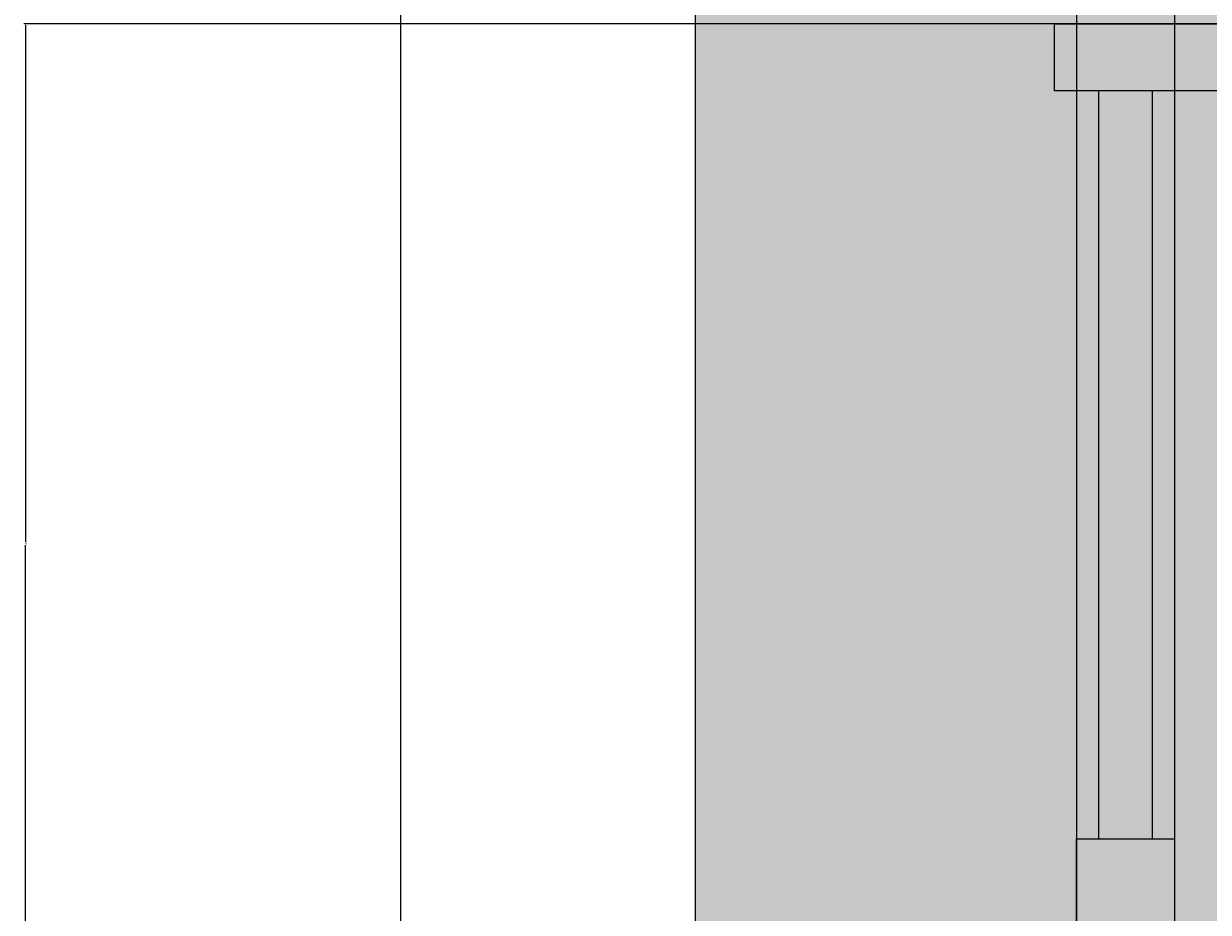
# Model space of a CAD drawing. Units: inches. Extents: x 3024 to 4744, y 1110 to 2100.
# Tile 3 of 29: x 3024 to 3168, y 1294 to 1402. Entities that reach past the tile are written whole.
import ezdxf

# ---------------------------------------------------------------- set-up
doc = ezdxf.new("R2010")
doc.units = ezdxf.units.IN
for name, color, linetype, lineweight in [('A-ANNO-DIMS', 2, 'Continuous', 18), ('A-ELEV', 7, 'Continuous', 25), ('A-ELEV-PATT', 252, 'Continuous', 13), ('A-GLAZ', 4, 'Continuous', 18)]:
    doc.layers.add(name, color=color, linetype=linetype, lineweight=lineweight)
doc.styles.get("Standard").update_dxf_attribs({"font": 'arial.ttf'})
doc.dimstyles.get("Standard").update_dxf_attribs({"dimtxt": 0.18, "dimasz": 0.18, "dimexe": 0.18, "dimexo": 0.0625, "dimgap": 0.09, "dimtad": 0, "dimtih": 1, "dimtoh": 1, "dimdec": 1, "dimzin": 0, "dimdsep": 46, "dimlunit": 3, "dimtxsty": 'Standard', "dimcen": 0.09, "dimadec": 0, "dimazin": 0, "dimtfac": 1, "dimtdec": 1, "dimtofl": 0, "dimtmove": 0, "dimatfit": 3, "dimfxl": 1, "dimtolj": 1, "dimtzin": 0, "dimarcsym": 0})

# ---------------------------------------------------------------- blocks, each defined once
blk = doc.blocks.new('WIN-BALCONY-A')
for p, q in [((3169.4, 1897.49), (3148.97, 1897.49)), ((3169.4, 1897.49), (3148.97, 1897.49)), ((3169.4, 1897.49), (3292.61, 1897.49)), ((3169.4, 1897.49), (3292.61, 1897.49)), ((3169.4, 1795.04), (3148.97, 1795.04)), ((3169.4, 1795.04), (3148.97, 1795.04)), ((3169.4, 1795.04), (3292.61, 1795.04)), ((3169.4, 1795.04), (3292.61, 1795.04))]:
    blk.add_line(p, q)
for points in [[(3148.97, 1897.49), (3148.97, 1905.61), (3292.61, 1905.61), (3292.61, 1897.49)], [(3148.97, 1897.49), (3148.97, 1905.61), (3292.61, 1905.61), (3292.61, 1897.49)], [(3292.61, 1795.04), (3292.61, 1785.61), (3148.97, 1785.61), (3148.97, 1795.04)], [(3292.61, 1795.04), (3292.61, 1785.61), (3148.97, 1785.61), (3148.97, 1795.04)]]:
    blk.add_lwpolyline(points)
for points in [[(3154.33, 1806.87), (3160.86, 1806.87), (3160.86, 1897.49), (3154.33, 1897.49)], [(3154.33, 1806.87), (3160.86, 1806.87), (3160.86, 1897.49), (3154.33, 1897.49)], [(3272.18, 1795.04), (3169.4, 1795.04), (3169.4, 1897.49), (3272.18, 1897.49)], [(3272.18, 1795.04), (3169.4, 1795.04), (3169.4, 1897.49), (3272.18, 1897.49)], [(3287.25, 1806.87), (3280.72, 1806.87), (3280.72, 1897.49), (3287.25, 1897.49)], [(3287.25, 1806.87), (3280.72, 1806.87), (3280.72, 1897.49), (3287.25, 1897.49)], [(3268.18, 1799.04), (3173.4, 1799.04), (3173.4, 1893.49), (3268.18, 1893.49)], [(3268.18, 1799.04), (3173.4, 1799.04), (3173.4, 1893.49), (3268.18, 1893.49)], [(3220.05, 1893.49), (3221.52, 1893.49), (3221.52, 1799.04), (3220.05, 1799.04)], [(3220.05, 1893.49), (3221.52, 1893.49), (3221.52, 1799.04), (3220.05, 1799.04)], [(3163.53, 1795.04), (3151.66, 1795.04), (3151.66, 1806.87), (3163.53, 1806.87)], [(3163.53, 1795.04), (3151.66, 1795.04), (3151.66, 1806.87), (3163.53, 1806.87)], [(3276.51, 1795.04), (3288.38, 1795.04), (3288.38, 1806.87), (3276.51, 1806.87)], [(3276.51, 1795.04), (3288.38, 1795.04), (3288.38, 1806.87), (3276.51, 1806.87)]]:
    blk.add_lwpolyline(points, close=True)
blk = doc.blocks.new('*D64')
at = {"layer": 'A-ANNO-DIMS', "color": 0, "lineweight": -2, "transparency": 16777216}
for p, q in [((3069.79, 1241.5), (3069.79, 2100.44)), ((3069.97, 2100.26), (3405.08, 2100.26)), ((3740.97, 2100.26), (3405.87, 2100.26)), ((3741.15, 1241.5), (3741.15, 2100.44))]:
    blk.add_line(p, q, dxfattribs=at)
at = {"layer": 'A-ANNO-DIMS', "color": 0, "transparency": 16777216}
for points in [[(3069.97, 2100.29), (3069.97, 2100.23), (3069.79, 2100.26)], [(3740.97, 2100.29), (3740.97, 2100.23), (3741.15, 2100.26)]]:
    blk.add_solid(points, dxfattribs=at)
at = {"layer": 'Defpoints', "color": 0, "transparency": 16777216}
for p in [(3741.15, 2100.26), (3069.79, 1241.43), (3741.15, 1241.43)]:
    blk.add_point(p, dxfattribs=at)
at = {"layer": 'A-ANNO-DIMS', "color": 0, "transparency": 16777216, "insert": (3405.47, 2100.26), "char_height": 0.18, "attachment_point": 5}
blk.add_mtext('\\A1;671.4', dxfattribs=at)
blk = doc.blocks.new('*D67')
at = {"layer": 'A-ANNO-DIMS', "color": 0, "lineweight": -2, "transparency": 16777216}
for p, q in [((3105.41, 1401.61), (3024.11, 1401.61)), ((3024.29, 1401.43), (3024.29, 1338.79)), ((3024.29, 1275.79), (3024.29, 1338.43)), ((3105.41, 1275.61), (3024.11, 1275.61))]:
    blk.add_line(p, q, dxfattribs=at)
at = {"layer": 'A-ANNO-DIMS', "color": 0, "transparency": 16777216}
for points in [[(3024.26, 1401.43), (3024.32, 1401.43), (3024.29, 1401.61)], [(3024.26, 1275.79), (3024.32, 1275.79), (3024.29, 1275.61)]]:
    blk.add_solid(points, dxfattribs=at)
at = {"layer": 'Defpoints', "color": 0, "transparency": 16777216}
for p in [(3024.29, 1401.61), (3105.47, 1401.61), (3105.47, 1275.61)]:
    blk.add_point(p, dxfattribs=at)
at = {"layer": 'A-ANNO-DIMS', "color": 0, "transparency": 16777216, "insert": (3024.29, 1338.61), "char_height": 0.18, "attachment_point": 5}
blk.add_mtext('\\A1;126', dxfattribs=at)
blk = doc.blocks.new('*D89')
at = {"layer": 'A-ANNO-DIMS', "color": 0, "lineweight": -2, "transparency": 16777216}
for p, q in [((3151.66, 1794.98), (3151.66, 1109.93)), ((3163.53, 1794.98), (3163.53, 1109.93)), ((3151.84, 1110.11), (3157.14, 1110.11)), ((3163.35, 1110.11), (3158.05, 1110.11))]:
    blk.add_line(p, q, dxfattribs=at)
at = {"layer": 'A-ANNO-DIMS', "color": 0, "transparency": 16777216}
for points in [[(3151.84, 1110.14), (3151.84, 1110.08), (3151.66, 1110.11)], [(3163.35, 1110.14), (3163.35, 1110.08), (3163.53, 1110.11)]]:
    blk.add_solid(points, dxfattribs=at)
at = {"layer": 'Defpoints', "color": 0, "transparency": 16777216}
for p in [(3151.66, 1795.04), (3163.53, 1795.04), (3163.53, 1110.11)]:
    blk.add_point(p, dxfattribs=at)
at = {"layer": 'A-ANNO-DIMS', "color": 0, "transparency": 16777216, "insert": (3157.59, 1110.11), "char_height": 0.18, "attachment_point": 5}
blk.add_mtext('\\A1;11.866', dxfattribs=at)

msp = doc.modelspace()

# ---------------------------------------------------------------- hatches: boundary and pattern name
at = {"layer": 'A-ELEV-PATT'}
h = msp.add_hatch(color=256, dxfattribs=at)
h.dxf.hatch_style = 1
h.paths.add_polyline_path([(3491.8271, 2054.7584), (3320.5658, 2054.7584), (3320.5658, 2043.5286), (3491.8271, 2043.5286)])
h.paths.add_polyline_path([(3292.6051, 1905.6112), (3148.9694, 1905.6112), (3148.9694, 1897.4879), (3169.3964, 1897.4879), (3292.6051, 1897.4879)])
h.paths.add_polyline_path([(3292.6051, 1795.0431), (3169.3964, 1795.0431), (3148.9694, 1795.0431), (3148.9694, 1785.6112), (3292.6051, 1785.6112)])
h.paths.add_polyline_path([(3292.6051, 1779.6112), (3148.9694, 1779.6112), (3148.9694, 1771.4879), (3169.3964, 1771.4879), (3292.6051, 1771.4879)])
h.paths.add_polyline_path([(3292.6051, 1669.0431), (3169.3964, 1669.0431), (3148.9694, 1669.0431), (3148.9694, 1659.6112), (3292.6051, 1659.6112)])
h.paths.add_polyline_path([(3292.6051, 1653.6112), (3148.9694, 1653.6112), (3148.9694, 1645.4879), (3169.3964, 1645.4879), (3292.6051, 1645.4879)])
h.paths.add_polyline_path([(3292.6051, 1543.0431), (3169.3964, 1543.0431), (3148.9694, 1543.0431), (3148.9694, 1533.6112), (3292.6051, 1533.6112)])
h.paths.add_polyline_path([(3292.6051, 1527.6112), (3148.9694, 1527.6112), (3148.9694, 1519.4879), (3169.3964, 1519.4879), (3292.6051, 1519.4879)])
h.paths.add_polyline_path([(3292.6051, 1401.6112), (3148.9694, 1401.6112), (3148.9694, 1393.4879), (3169.3964, 1393.4879), (3292.6051, 1393.4879)])
h.paths.add_polyline_path([(3292.6051, 1417.0431), (3169.3964, 1417.0431), (3148.9694, 1417.0431), (3148.9694, 1407.6112), (3292.6051, 1407.6112)])
h.paths.add_polyline_path([(3292.6051, 1291.0431), (3169.3964, 1291.0431), (3148.9694, 1291.0431), (3148.9694, 1281.6112), (3292.6051, 1281.6112)])
h.paths.add_polyline_path([(3654.037, 1165.0431), (3530.8283, 1165.0431), (3510.4013, 1165.0431), (3510.4013, 1155.6112), (3654.037, 1155.6112)])
h.paths.add_polyline_path([(3654.037, 1275.6112), (3510.4013, 1275.6112), (3510.4013, 1267.4879), (3530.8283, 1267.4879), (3654.037, 1267.4879)])
h.paths.add_polyline_path([(3654.037, 1291.0431), (3530.8283, 1291.0431), (3510.4013, 1291.0431), (3510.4013, 1281.6112), (3654.037, 1281.6112)])
h.paths.add_polyline_path([(3654.037, 1417.0431), (3530.8283, 1417.0431), (3510.4013, 1417.0431), (3510.4013, 1407.6112), (3654.037, 1407.6112)])
h.paths.add_polyline_path([(3654.037, 1401.6112), (3510.4013, 1401.6112), (3510.4013, 1393.4879), (3530.8283, 1393.4879), (3654.037, 1393.4879)])
h.paths.add_polyline_path([(3654.037, 1543.0431), (3530.8283, 1543.0431), (3510.4013, 1543.0431), (3510.4013, 1533.6112), (3654.037, 1533.6112)])
h.paths.add_polyline_path([(3654.037, 1527.6112), (3510.4013, 1527.6112), (3510.4013, 1519.4879), (3530.8283, 1519.4879), (3654.037, 1519.4879)])
h.paths.add_polyline_path([(3654.037, 1653.6112), (3510.4013, 1653.6112), (3510.4013, 1645.4879), (3530.8283, 1645.4879), (3654.037, 1645.4879)])
h.paths.add_polyline_path([(3654.037, 1669.0431), (3530.8283, 1669.0431), (3510.4013, 1669.0431), (3510.4013, 1659.6112), (3654.037, 1659.6112)])
h.paths.add_polyline_path([(3654.037, 1779.6112), (3510.4013, 1779.6112), (3510.4013, 1771.4879), (3530.8283, 1771.4879), (3654.037, 1771.4879)])
h.paths.add_polyline_path([(3654.037, 1795.0431), (3530.8283, 1795.0431), (3510.4013, 1795.0431), (3510.4013, 1785.6112), (3654.037, 1785.6112)])
h.paths.add_polyline_path([(3654.037, 1905.6112), (3510.4013, 1905.6112), (3510.4013, 1897.4879), (3530.8283, 1897.4879), (3654.037, 1897.4879)])
h = msp.add_hatch(color=256, dxfattribs=at)
h.dxf.hatch_style = 1
h.paths.add_polyline_path([(3329.7033, 1407.6112), (3105.4722, 1407.6112), (3105.4722, 1401.6112), (3329.7033, 1401.6112)])
h.paths.add_polyline_path([(3329.7033, 1281.6112), (3105.4722, 1281.6112), (3105.4722, 1275.6112), (3112.3838, 1275.6112), (3329.7033, 1275.6112)])
h.paths.add_polyline_path([(3329.7033, 1533.6112), (3105.4722, 1533.6112), (3105.4722, 1527.6112), (3329.7033, 1527.6112)])
h.paths.add_polyline_path([(3329.7033, 1659.6112), (3105.4722, 1659.6112), (3105.4722, 1653.6112), (3329.7033, 1653.6112)])
h.paths.add_polyline_path([(3329.7033, 1785.6112), (3105.4722, 1785.6112), (3105.4722, 1779.6112), (3329.7033, 1779.6112)])
h.paths.add_polyline_path([(3329.7033, 1911.6112), (3105.4722, 1911.6112), (3095.7158, 1911.6112), (3095.7158, 1905.6112), (3329.7033, 1905.6112)])
h.paths.add_polyline_path([(3715.2286, 1911.6112), (3705.4722, 1911.6112), (3705.4722, 1905.6112), (3715.2286, 1905.6112)])
h.paths.add_polyline_path([(3688.5588, 1911.6112), (3481.2411, 1911.6112), (3481.2411, 1905.6112), (3688.5588, 1905.6112)])
h = msp.add_hatch(color=256, dxfattribs=at)
h.dxf.hatch_style = 1
h.paths.add_polyline_path([(3154.3287, 1897.4879), (3148.9694, 1897.4879), (3148.9694, 1905.6112), (3105.4722, 1905.6112), (3105.4722, 1785.6112), (3148.9694, 1785.6112), (3148.9694, 1795.0431), (3151.6604, 1795.0431), (3151.6604, 1806.8674), (3154.3287, 1806.8674)])
h.paths.add_polyline_path([(3329.7033, 1905.6112), (3292.6051, 1905.6112), (3292.6051, 1897.4879), (3287.2458, 1897.4879), (3287.2458, 1806.8674), (3288.3759, 1806.8674), (3288.3759, 1795.0431), (3292.6051, 1795.0431), (3292.6051, 1785.6112), (3329.7033, 1785.6112)])
h.paths.add_polyline_path([(3154.3287, 1771.4879), (3148.9694, 1771.4879), (3148.9694, 1779.6112), (3105.4722, 1779.6112), (3105.4722, 1659.6112), (3148.9694, 1659.6112), (3148.9694, 1669.0431), (3151.6604, 1669.0431), (3151.6604, 1680.8674), (3154.3287, 1680.8674)])
h.paths.add_polyline_path([(3329.7033, 1779.6112), (3292.6051, 1779.6112), (3292.6051, 1771.4879), (3287.2458, 1771.4879), (3287.2458, 1680.8674), (3288.3759, 1680.8674), (3288.3759, 1669.0431), (3292.6051, 1669.0431), (3292.6051, 1659.6112), (3329.7033, 1659.6112)])
h.paths.add_polyline_path([(3154.3287, 1645.4879), (3148.9694, 1645.4879), (3148.9694, 1653.6112), (3105.4722, 1653.6112), (3105.4722, 1533.6112), (3148.9694, 1533.6112), (3148.9694, 1543.0431), (3151.6604, 1543.0431), (3151.6604, 1554.8674), (3154.3287, 1554.8674)])
h.paths.add_polyline_path([(3329.7033, 1653.6112), (3292.6051, 1653.6112), (3292.6051, 1645.4879), (3287.2458, 1645.4879), (3287.2458, 1554.8674), (3288.3759, 1554.8674), (3288.3759, 1543.0431), (3292.6051, 1543.0431), (3292.6051, 1533.6112), (3329.7033, 1533.6112)])
h.paths.add_polyline_path([(3329.7033, 1527.6112), (3292.6051, 1527.6112), (3292.6051, 1519.4879), (3287.2458, 1519.4879), (3287.2458, 1428.8674), (3288.3759, 1428.8674), (3288.3759, 1417.0431), (3292.6051, 1417.0431), (3292.6051, 1407.6112), (3329.7033, 1407.6112)])
h.paths.add_polyline_path([(3329.7033, 1401.6112), (3292.6051, 1401.6112), (3292.6051, 1393.4879), (3287.2458, 1393.4879), (3287.2458, 1302.8674), (3288.3759, 1302.8674), (3288.3759, 1291.0431), (3292.6051, 1291.0431), (3292.6051, 1281.6112), (3329.7033, 1281.6112)])
h.paths.add_polyline_path([(3154.3287, 1393.4879), (3148.9694, 1393.4879), (3148.9694, 1401.6112), (3105.4722, 1401.6112), (3105.4722, 1281.6112), (3148.9694, 1281.6112), (3148.9694, 1291.0431), (3151.6604, 1291.0431), (3151.6604, 1302.8674), (3154.3287, 1302.8674)])
h.paths.add_polyline_path([(3154.3287, 1519.4879), (3148.9694, 1519.4879), (3148.9694, 1527.6112), (3105.4722, 1527.6112), (3105.4722, 1407.6112), (3148.9694, 1407.6112), (3148.9694, 1417.0431), (3151.6604, 1417.0431), (3151.6604, 1428.8674), (3154.3287, 1428.8674)])
h.paths.add_polyline_path([(3515.7606, 1897.4879), (3510.4013, 1897.4879), (3510.4013, 1905.6112), (3481.2411, 1905.6112), (3481.2411, 1785.6112), (3510.4013, 1785.6112), (3510.4013, 1795.0431), (3513.0923, 1795.0431), (3513.0923, 1806.8674), (3515.7606, 1806.8674)])
h.paths.add_polyline_path([(3688.5588, 1905.6112), (3654.037, 1905.6112), (3654.037, 1897.4879), (3648.6777, 1897.4879), (3648.6777, 1806.8674), (3649.8078, 1806.8674), (3649.8078, 1795.0431), (3654.037, 1795.0431), (3654.037, 1785.6112), (3688.5588, 1785.6112)])
h.paths.add_polyline_path([(3515.7606, 1771.4879), (3510.4013, 1771.4879), (3510.4013, 1779.6112), (3481.2411, 1779.6112), (3481.2411, 1659.6112), (3510.4013, 1659.6112), (3510.4013, 1669.0431), (3513.0923, 1669.0431), (3513.0923, 1680.8674), (3515.7606, 1680.8674)])
h.paths.add_polyline_path([(3688.5588, 1779.6112), (3654.037, 1779.6112), (3654.037, 1771.4879), (3648.6777, 1771.4879), (3648.6777, 1680.8674), (3649.8078, 1680.8674), (3649.8078, 1669.0431), (3654.037, 1669.0431), (3654.037, 1659.6112), (3688.5588, 1659.6112)])
h.paths.add_polyline_path([(3515.7606, 1645.4879), (3510.4013, 1645.4879), (3510.4013, 1653.6112), (3481.2411, 1653.6112), (3481.2411, 1533.6112), (3510.4013, 1533.6112), (3510.4013, 1543.0431), (3513.0923, 1543.0431), (3513.0923, 1554.8674), (3515.7606, 1554.8674)])
h.paths.add_polyline_path([(3688.5588, 1653.6112), (3654.037, 1653.6112), (3654.037, 1645.4879), (3648.6777, 1645.4879), (3648.6777, 1554.8674), (3649.8078, 1554.8674), (3649.8078, 1543.0431), (3654.037, 1543.0431), (3654.037, 1533.6112), (3688.5588, 1533.6112)])
h.paths.add_polyline_path([(3515.7606, 1519.4879), (3510.4013, 1519.4879), (3510.4013, 1527.6112), (3481.2411, 1527.6112), (3481.2411, 1407.6112), (3510.4013, 1407.6112), (3510.4013, 1417.0431), (3513.0923, 1417.0431), (3513.0923, 1428.8674), (3515.7606, 1428.8674)])
h.paths.add_polyline_path([(3688.5588, 1527.6112), (3654.037, 1527.6112), (3654.037, 1519.4879), (3648.6777, 1519.4879), (3648.6777, 1428.8674), (3649.8078, 1428.8674), (3649.8078, 1417.0431), (3654.037, 1417.0431), (3654.037, 1407.6112), (3688.5588, 1407.6112)])
h.paths.add_polyline_path([(3515.7606, 1393.4879), (3510.4013, 1393.4879), (3510.4013, 1401.6112), (3481.2411, 1401.6112), (3481.2411, 1281.6112), (3510.4013, 1281.6112), (3510.4013, 1291.0431), (3513.0923, 1291.0431), (3513.0923, 1302.8674), (3515.7606, 1302.8674)])
h.paths.add_polyline_path([(3688.5588, 1401.6112), (3654.037, 1401.6112), (3654.037, 1393.4879), (3648.6777, 1393.4879), (3648.6777, 1302.8674), (3649.8078, 1302.8674), (3649.8078, 1291.0431), (3654.037, 1291.0431), (3654.037, 1281.6112), (3688.5588, 1281.6112)])
h.paths.add_polyline_path([(3515.7606, 1267.4879), (3510.4013, 1267.4879), (3510.4013, 1275.6112), (3481.2411, 1275.6112), (3481.2411, 1155.6112), (3510.4013, 1155.6112), (3510.4013, 1165.0431), (3513.0923, 1165.0431), (3513.0923, 1176.8674), (3515.7606, 1176.8674)])
h.paths.add_polyline_path([(3688.5588, 1275.6112), (3654.037, 1275.6112), (3654.037, 1267.4879), (3648.6777, 1267.4879), (3648.6777, 1176.8674), (3649.8078, 1176.8674), (3649.8078, 1165.0431), (3654.037, 1165.0431), (3654.037, 1155.6112), (3688.5588, 1155.6112)])
h.paths.add_polyline_path([(3112.3838, 1275.6112), (3105.4722, 1275.6112), (3105.4722, 1171.0239), (3112.3838, 1171.0239)])
h = msp.add_hatch(color=256, dxfattribs=at)
h.dxf.hatch_style = 1
h.paths.add_polyline_path([(3160.8586, 1897.4879), (3154.3287, 1897.4879), (3154.3287, 1806.8674), (3160.8586, 1806.8674)])
h.paths.add_polyline_path([(3287.2458, 1897.4879), (3280.716, 1897.4879), (3280.716, 1806.8674), (3287.2458, 1806.8674)])
h.paths.add_polyline_path([(3160.8586, 1771.4879), (3154.3287, 1771.4879), (3154.3287, 1680.8674), (3160.8586, 1680.8674)])
h.paths.add_polyline_path([(3287.2458, 1771.4879), (3280.716, 1771.4879), (3280.716, 1680.8674), (3287.2458, 1680.8674)])
h.paths.add_polyline_path([(3160.8586, 1645.4879), (3154.3287, 1645.4879), (3154.3287, 1554.8674), (3160.8586, 1554.8674)])
h.paths.add_polyline_path([(3287.2458, 1645.4879), (3280.716, 1645.4879), (3280.716, 1554.8674), (3287.2458, 1554.8674)])
h.paths.add_polyline_path([(3160.8586, 1519.4879), (3154.3287, 1519.4879), (3154.3287, 1428.8674), (3160.8586, 1428.8674)])
h.paths.add_polyline_path([(3287.2458, 1519.4879), (3280.716, 1519.4879), (3280.716, 1428.8674), (3287.2458, 1428.8674)])
h.paths.add_polyline_path([(3160.8586, 1393.4879), (3154.3287, 1393.4879), (3154.3287, 1302.8674), (3160.8586, 1302.8674)])
h.paths.add_polyline_path([(3287.2458, 1393.4879), (3280.716, 1393.4879), (3280.716, 1302.8674), (3287.2458, 1302.8674)])
h.paths.add_polyline_path([(3648.6777, 1267.4879), (3642.1479, 1267.4879), (3642.1479, 1176.8674), (3648.6777, 1176.8674)])
h.paths.add_polyline_path([(3522.2905, 1267.4879), (3515.7606, 1267.4879), (3515.7606, 1176.8674), (3522.2905, 1176.8674)])
h.paths.add_polyline_path([(3522.2905, 1393.4879), (3515.7606, 1393.4879), (3515.7606, 1302.8674), (3522.2905, 1302.8674)])
h.paths.add_polyline_path([(3648.6777, 1393.4879), (3642.1479, 1393.4879), (3642.1479, 1302.8674), (3648.6777, 1302.8674)])
h.paths.add_polyline_path([(3522.2905, 1519.4879), (3515.7606, 1519.4879), (3515.7606, 1428.8674), (3522.2905, 1428.8674)])
h.paths.add_polyline_path([(3648.6777, 1519.4879), (3642.1479, 1519.4879), (3642.1479, 1428.8674), (3648.6777, 1428.8674)])
h.paths.add_polyline_path([(3522.2905, 1645.4879), (3515.7606, 1645.4879), (3515.7606, 1554.8674), (3522.2905, 1554.8674)])
h.paths.add_polyline_path([(3522.2905, 1771.4879), (3515.7606, 1771.4879), (3515.7606, 1680.8674), (3522.2905, 1680.8674)])
h.paths.add_polyline_path([(3648.6777, 1645.4879), (3642.1479, 1645.4879), (3642.1479, 1554.8674), (3648.6777, 1554.8674)])
h.paths.add_polyline_path([(3648.6777, 1771.4879), (3642.1479, 1771.4879), (3642.1479, 1680.8674), (3648.6777, 1680.8674)])
h.paths.add_polyline_path([(3648.6777, 1897.4879), (3642.1479, 1897.4879), (3642.1479, 1806.8674), (3648.6777, 1806.8674)])
h.paths.add_polyline_path([(3522.2905, 1897.4879), (3515.7606, 1897.4879), (3515.7606, 1806.8674), (3522.2905, 1806.8674)])
h = msp.add_hatch(color=256, dxfattribs=at)
h.dxf.hatch_style = 1
h.paths.add_polyline_path([(3169.3964, 1897.4879), (3160.8586, 1897.4879), (3160.8586, 1806.8674), (3163.5269, 1806.8674), (3163.5269, 1795.0431), (3169.3964, 1795.0431)])
h.paths.add_polyline_path([(3280.716, 1897.4879), (3272.1781, 1897.4879), (3272.1781, 1795.0431), (3276.5094, 1795.0431), (3276.5094, 1806.8674), (3280.716, 1806.8674)])
h.paths.add_polyline_path([(3280.716, 1771.4879), (3272.1781, 1771.4879), (3272.1781, 1669.0431), (3276.5094, 1669.0431), (3276.5094, 1680.8674), (3280.716, 1680.8674)])
h.paths.add_polyline_path([(3169.3964, 1771.4879), (3160.8586, 1771.4879), (3160.8586, 1680.8674), (3163.5269, 1680.8674), (3163.5269, 1669.0431), (3169.3964, 1669.0431)])
h.paths.add_polyline_path([(3169.3964, 1645.4879), (3160.8586, 1645.4879), (3160.8586, 1554.8674), (3163.5269, 1554.8674), (3163.5269, 1543.0431), (3169.3964, 1543.0431)])
h.paths.add_polyline_path([(3280.716, 1645.4879), (3272.1781, 1645.4879), (3272.1781, 1543.0431), (3276.5094, 1543.0431), (3276.5094, 1554.8674), (3280.716, 1554.8674)])
h.paths.add_polyline_path([(3169.3964, 1519.4879), (3160.8586, 1519.4879), (3160.8586, 1428.8674), (3163.5269, 1428.8674), (3163.5269, 1417.0431), (3169.3964, 1417.0431)])
h.paths.add_polyline_path([(3280.716, 1519.4879), (3272.1781, 1519.4879), (3272.1781, 1417.0431), (3276.5094, 1417.0431), (3276.5094, 1428.8674), (3280.716, 1428.8674)])
h.paths.add_polyline_path([(3169.3964, 1393.4879), (3160.8586, 1393.4879), (3160.8586, 1302.8674), (3163.5269, 1302.8674), (3163.5269, 1291.0431), (3169.3964, 1291.0431)])
h.paths.add_polyline_path([(3280.716, 1393.4879), (3272.1781, 1393.4879), (3272.1781, 1291.0431), (3276.5094, 1291.0431), (3276.5094, 1302.8674), (3280.716, 1302.8674)])
h.paths.add_polyline_path([(3642.1479, 1267.4879), (3633.61, 1267.4879), (3633.61, 1165.0431), (3637.9413, 1165.0431), (3637.9413, 1176.8674), (3642.1479, 1176.8674)])
h.paths.add_polyline_path([(3530.8283, 1267.4879), (3522.2905, 1267.4879), (3522.2905, 1176.8674), (3524.9588, 1176.8674), (3524.9588, 1165.0431), (3530.8283, 1165.0431)])
h.paths.add_polyline_path([(3642.1479, 1393.4879), (3633.61, 1393.4879), (3633.61, 1291.0431), (3637.9413, 1291.0431), (3637.9413, 1302.8674), (3642.1479, 1302.8674)])
h.paths.add_polyline_path([(3530.8283, 1393.4879), (3522.2905, 1393.4879), (3522.2905, 1302.8674), (3524.9588, 1302.8674), (3524.9588, 1291.0431), (3530.8283, 1291.0431)])
h.paths.add_polyline_path([(3530.8283, 1519.4879), (3522.2905, 1519.4879), (3522.2905, 1428.8674), (3524.9588, 1428.8674), (3524.9588, 1417.0431), (3530.8283, 1417.0431)])
h.paths.add_polyline_path([(3642.1479, 1519.4879), (3633.61, 1519.4879), (3633.61, 1417.0431), (3637.9413, 1417.0431), (3637.9413, 1428.8674), (3642.1479, 1428.8674)])
h.paths.add_polyline_path([(3530.8283, 1645.4879), (3522.2905, 1645.4879), (3522.2905, 1554.8674), (3524.9588, 1554.8674), (3524.9588, 1543.0431), (3530.8283, 1543.0431)])
h.paths.add_polyline_path([(3642.1479, 1645.4879), (3633.61, 1645.4879), (3633.61, 1543.0431), (3637.9413, 1543.0431), (3637.9413, 1554.8674), (3642.1479, 1554.8674)])
h.paths.add_polyline_path([(3642.1479, 1771.4879), (3633.61, 1771.4879), (3633.61, 1669.0431), (3637.9413, 1669.0431), (3637.9413, 1680.8674), (3642.1479, 1680.8674)])
h.paths.add_polyline_path([(3530.8283, 1771.4879), (3522.2905, 1771.4879), (3522.2905, 1680.8674), (3524.9588, 1680.8674), (3524.9588, 1669.0431), (3530.8283, 1669.0431)])
h.paths.add_polyline_path([(3530.8283, 1897.4879), (3522.2905, 1897.4879), (3522.2905, 1806.8674), (3524.9588, 1806.8674), (3524.9588, 1795.0431), (3530.8283, 1795.0431)])
h.paths.add_polyline_path([(3642.1479, 1897.4879), (3633.61, 1897.4879), (3633.61, 1795.0431), (3637.9413, 1795.0431), (3637.9413, 1806.8674), (3642.1479, 1806.8674)])
h = msp.add_hatch(color=256, dxfattribs=at)
h.dxf.hatch_style = 1
h.paths.add_polyline_path([(3163.5269, 1302.8674), (3151.6604, 1302.8674), (3151.6604, 1291.0431), (3163.5269, 1291.0431)])
h.paths.add_polyline_path([(3288.3759, 1302.8674), (3276.5094, 1302.8674), (3276.5094, 1291.0431), (3288.3759, 1291.0431)])
h.paths.add_polyline_path([(3288.3759, 1428.8674), (3276.5094, 1428.8674), (3276.5094, 1417.0431), (3288.3759, 1417.0431)])
h.paths.add_polyline_path([(3163.5269, 1428.8674), (3151.6604, 1428.8674), (3151.6604, 1417.0431), (3163.5269, 1417.0431)])
h.paths.add_polyline_path([(3163.5269, 1554.8674), (3151.6604, 1554.8674), (3151.6604, 1543.0431), (3163.5269, 1543.0431)])
h.paths.add_polyline_path([(3288.3759, 1554.8674), (3276.5094, 1554.8674), (3276.5094, 1543.0431), (3288.3759, 1543.0431)])
h.paths.add_polyline_path([(3163.5269, 1680.8674), (3151.6604, 1680.8674), (3151.6604, 1669.0431), (3163.5269, 1669.0431)])
h.paths.add_polyline_path([(3288.3759, 1680.8674), (3276.5094, 1680.8674), (3276.5094, 1669.0431), (3288.3759, 1669.0431)])
h.paths.add_polyline_path([(3163.5269, 1806.8674), (3151.6604, 1806.8674), (3151.6604, 1795.0431), (3163.5269, 1795.0431)])
h.paths.add_polyline_path([(3288.3759, 1806.8674), (3276.5094, 1806.8674), (3276.5094, 1795.0431), (3288.3759, 1795.0431)])
h.paths.add_polyline_path([(3524.9588, 1806.8674), (3513.0923, 1806.8674), (3513.0923, 1795.0431), (3524.9588, 1795.0431)])
h.paths.add_polyline_path([(3649.8078, 1806.8674), (3637.9413, 1806.8674), (3637.9413, 1795.0431), (3649.8078, 1795.0431)])
h.paths.add_polyline_path([(3524.9588, 1680.8674), (3513.0923, 1680.8674), (3513.0923, 1669.0431), (3524.9588, 1669.0431)])
h.paths.add_polyline_path([(3649.8078, 1680.8674), (3637.9413, 1680.8674), (3637.9413, 1669.0431), (3649.8078, 1669.0431)])
h.paths.add_polyline_path([(3524.9588, 1554.8674), (3513.0923, 1554.8674), (3513.0923, 1543.0431), (3524.9588, 1543.0431)])
h.paths.add_polyline_path([(3649.8078, 1554.8674), (3637.9413, 1554.8674), (3637.9413, 1543.0431), (3649.8078, 1543.0431)])
h.paths.add_polyline_path([(3524.9588, 1428.8674), (3513.0923, 1428.8674), (3513.0923, 1417.0431), (3524.9588, 1417.0431)])
h.paths.add_polyline_path([(3649.8078, 1428.8674), (3637.9413, 1428.8674), (3637.9413, 1417.0431), (3649.8078, 1417.0431)])
h.paths.add_polyline_path([(3524.9588, 1302.8674), (3513.0923, 1302.8674), (3513.0923, 1291.0431), (3524.9588, 1291.0431)])
h.paths.add_polyline_path([(3649.8078, 1302.8674), (3637.9413, 1302.8674), (3637.9413, 1291.0431), (3649.8078, 1291.0431)])
h.paths.add_polyline_path([(3524.9588, 1176.8674), (3513.0923, 1176.8674), (3513.0923, 1165.0431), (3524.9588, 1165.0431)])
h.paths.add_polyline_path([(3649.8078, 1176.8674), (3637.9413, 1176.8674), (3637.9413, 1165.0431), (3649.8078, 1165.0431)])

# ---------------------------------------------------------------- linework, layer by layer
at = {"layer": 'A-ELEV'}
for p, q in [((3105.4722, 1171.0239), (3105.4722, 1905.6112)), ((3105.4722, 1171.0239), (3105.4722, 1905.6112)), ((3329.7033, 1401.6112), (3105.4722, 1401.6112)), ((3329.7033, 1401.6112), (3105.4722, 1401.6112))]:
    msp.add_line(p, q, dxfattribs=at)

# ---------------------------------------------------------------- block references
at = {"layer": 'A-GLAZ'}
msp.add_blockref('WIN-BALCONY-A', (0, -504), dxfattribs=at)

# ---------------------------------------------------------------- dimensions: what is measured, and where the dimension line sits
at = {"layer": 'A-ANNO-DIMS'}
for base, p1, p2, override, picture, middle in [((3741.1507, 2100.2584), (3069.7937, 1241.4341), (3741.1507, 1241.4341), {"dimdec": 1, "dimlfac": 1, "dimrnd": 0, "dimzin": 0, "dimdsep": 46, "dimlunit": 2}, '*D64', (3405.4722, 2100.2584)), ((3163.526875, 1110.111173), (3151.660378, 1795.043127), (3163.526875, 1795.043127), {"dimdec": 3, "dimlfac": 1, "dimrnd": 0, "dimzin": 0, "dimdsep": 46, "dimlunit": 2}, '*D89', (3157.593627, 1110.111173))]:
    dim = msp.add_linear_dim(base=base, p1=p1, p2=p2, dimstyle='Standard', override=override, dxfattribs=at)
    dim.commit()
    dim.dimension.update_dxf_attribs({"geometry": picture, "text_midpoint": middle})
dim = msp.add_linear_dim(base=(3024.2937, 1401.6112), p1=(3105.4722, 1275.6112), p2=(3105.4722, 1401.6112), angle=90, dimstyle='Standard', override={"dimdec": 0, "dimlfac": 1, "dimrnd": 0, "dimzin": 0, "dimdsep": 46, "dimlunit": 2}, dxfattribs=at)
dim.commit()
dim.dimension.update_dxf_attribs({"geometry": '*D67', "text_midpoint": (3024.2937, 1338.6112)})

doc.saveas('drawing.dxf')
